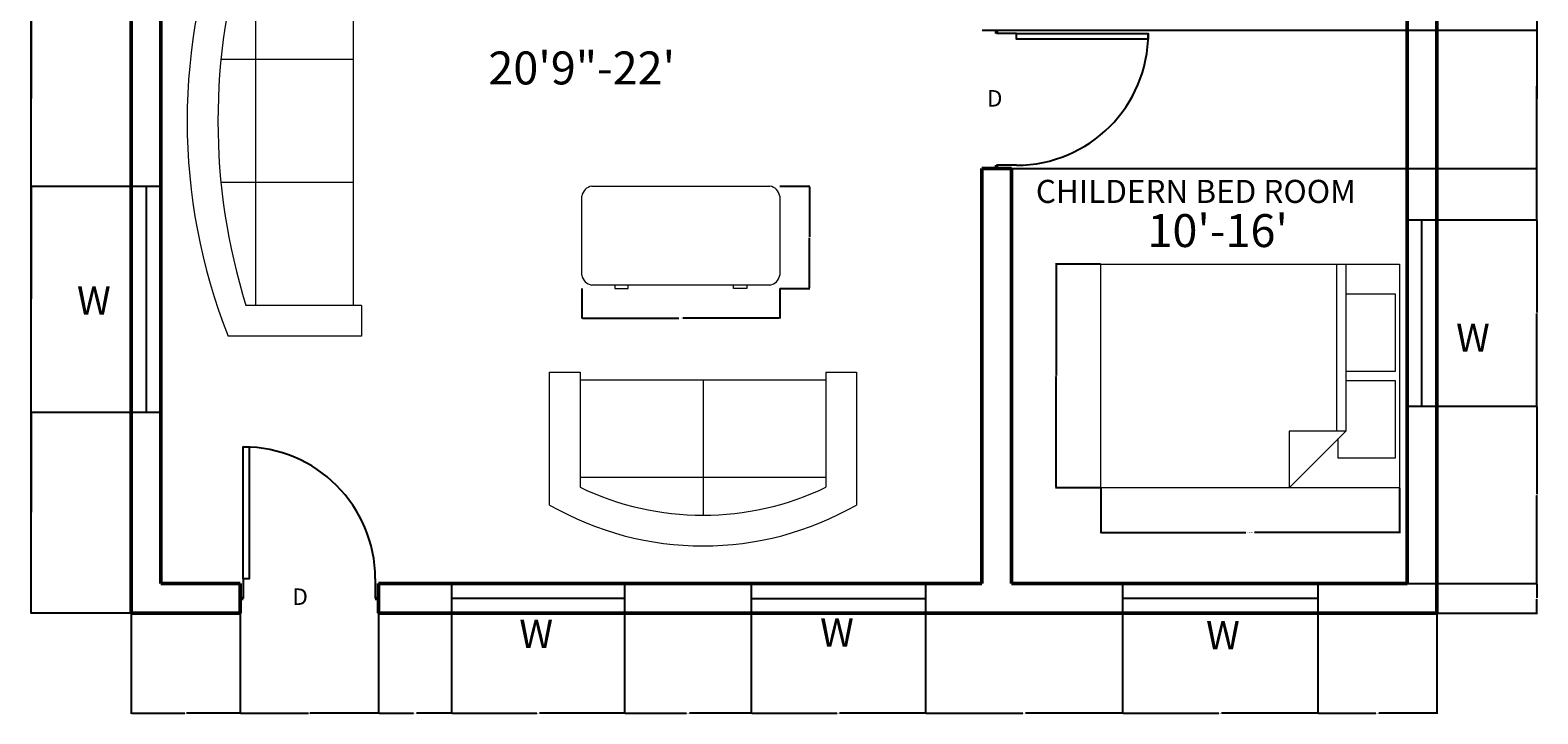
# Model space of a CAD drawing. Units: inches. Extents: x 2164 to 3752, y 2015 to 2629.
# Tile 1 of 8: x 2164 to 2622, y 2015 to 2223. Entities that reach past the tile are written whole.
import ezdxf
from ezdxf.enums import TextEntityAlignment as Align

# ---------------------------------------------------------------- set-up
doc = ezdxf.new("R2010")
doc.units = ezdxf.units.IN
for name, color, linetype, lineweight in [('A-ANNO-DIMS', 2, 'Continuous', 18), ('A-ANNO-TEXT', 7, 'Continuous', 25), ('A-AREA-IDEN', 3, 'Continuous', 25), ('A-DOOR', 3, 'Continuous', 25), ('A-FURN', 8, 'Continuous', 18), ('A-GLAZ', 4, 'Continuous', 25), ('A-WALL', 7, 'Continuous', 50)]:
    doc.layers.add(name, color=color, linetype=linetype, lineweight=lineweight)
doc.styles.get("Standard").update_dxf_attribs({"font": 'arial.ttf'})
doc.dimstyles.get("Standard").update_dxf_attribs({"dimtxt": 0.18, "dimasz": 0.18, "dimexe": 0.18, "dimexo": 0.0625, "dimgap": 0.09, "dimtad": 0, "dimtih": 1, "dimtoh": 1, "dimdec": 4, "dimzin": 0, "dimdsep": 46, "dimtxsty": 'Standard', "dimcen": 0.09, "dimadec": 0, "dimazin": 0, "dimtfac": 1, "dimtdec": 4, "dimtofl": 0, "dimtmove": 0, "dimatfit": 3, "dimfxl": 1, "dimtolj": 1, "dimtzin": 0, "dimarcsym": 0})

# ---------------------------------------------------------------- blocks, each defined once
blk = doc.blocks.new('*U7')
for p, q in [((0, 0), (0, -6)), ((40, 0), (40, -6))]:
    blk.add_line(p, q)
blk.add_lwpolyline([(0, 0), (0, 40), (1.75, 40), (1.75, 0)], close=True)
blk.add_arc((0, 0), 40, 0, 90)
blk = doc.blocks.new('Sofa - Roundback 7 ft.')
for p, q in [((-12.00002, -32.4421), (-12.00003, -6.5971)), ((11.99997, -32.4421), (11.99998, -6.5971)), ((-36.000027, -34), (-36.000027, -11.4696)), ((35.99998, -34), (35.99998, -11.4696)), ((-35.999844, -13.3819), (35.9998, -13.3819)), ((-36.000027, -32.4421), (35.99998, -32.4421))]:
    blk.add_line(p, q)
for points in [[(-36.000027, -34), (-42.000027, -34), (-42.000027, -8)], [(41.99998, -8), (41.99998, -34), (35.99998, -34)]]:
    blk.add_lwpolyline(points)
for centre, radius, start, end in [((0, -114.25), 114.25, 68.43141, 111.5686), ((-0.00001, -127.1968), 121.1968, 72.72033, 107.2797)]:
    blk.add_arc(centre, radius, start, end)
blk = doc.blocks.new('Sofa - Roundback Loveseat 5 ft.')
for p, q in [((0, -32.44198), (0, -5.99998)), ((-24, -33.99998), (-24, -11.46958)), ((24.00004, -33.99998), (24.00004, -11.46958)), ((-23.9998, -13.38178), (23.99986, -13.38178)), ((-24, -32.44198), (24.00004, -32.44198))]:
    blk.add_line(p, q)
for points in [[(-24, -33.99998), (-30, -33.99998), (-30, -7.99998)], [(30.00004, -7.99998), (30.00004, -33.99998), (24.00004, -33.99998)]]:
    blk.add_lwpolyline(points)
for centre, radius, start, end in [((0, -60.24998), 60.24998, 60.13715, 119.8628), ((0, -61.38438), 55.38444, 64.32083, 115.6792)]:
    blk.add_arc(centre, radius, start, end)
blk = doc.blocks.new('Bed - Queen')
for p, q in [((0, -80.00003), (0, 0)), ((0, 0), (59.99999, 0)), ((59.99999, 0), (59.99999, -80.00003)), ((7.99999, -1.2), (28.79998, -1.2)), ((7.99999, -14.4), (7.99999, -1.2)), ((28.79998, -1.2), (28.79998, -14.4)), ((31.19999, -1.2), (51.99999, -1.2)), ((31.19999, -14.4), (31.19999, -1.2)), ((51.99999, -1.2), (51.99999, -16.4)), ((0, -14.4), (44.8, -14.4)), ((59.99999, -29.6), (44.8, -14.4)), ((44.8, -14.4), (44.8, -29.6)), ((44.8, -16.8), (0, -16.8)), ((51.99999, -16.4), (46.79936, -16.4)), ((44.8, -29.6), (59.99999, -29.6)), ((59.99999, -80.00003), (0, -80.00003))]:
    blk.add_line(p, q)
blk = doc.blocks.new('Desk - 30 x 60 in.')
for p, q in [((-26.999995, 0), (26.999995, 0)), ((-29.999995, -27), (-29.999995, -3)), ((29.999995, -3), (29.999995, -27)), ((26.999995, -30), (-26.999995, -30)), ((-20.000005, -30), (-20.000005, -31)), ((-20.000005, -31), (-16.000005, -31)), ((-16.000005, -31), (-16.000005, -30)), ((15.999995, -31), (15.999995, -30)), ((19.999995, -31), (15.999995, -31)), ((19.999995, -30), (19.999995, -31))]:
    blk.add_line(p, q)
for centre, start, end in [((-26.499995, -3.5), 98.1301, 171.8699), ((26.499995, -3.5), 8.130102, 81.8699), ((-26.499995, -26.5), 188.1301, 261.8699), ((26.499995, -26.5), 278.1301, 351.8699)]:
    blk.add_arc(centre, 3.535534, start, end)
blk = doc.blocks.new('*D21')
at = {"layer": 'A-ANNO-DIMS', "color": 0, "lineweight": -2, "transparency": 16777216}
for p, q in [((2489.23, 2083.72), (2489.23, 2070.01)), ((2579.81, 2083.72), (2579.81, 2070.01)), ((2489.41, 2070.19), (2533.21, 2070.19)), ((2579.63, 2070.19), (2535.82, 2070.19))]:
    blk.add_line(p, q, dxfattribs=at)
at = {"layer": 'A-ANNO-DIMS', "color": 0, "transparency": 16777216}
for points in [[(2489.41, 2070.22), (2489.41, 2070.16), (2489.23, 2070.19)], [(2579.63, 2070.22), (2579.63, 2070.16), (2579.81, 2070.19)]]:
    blk.add_solid(points, dxfattribs=at)
at = {"layer": 'Defpoints', "color": 0, "transparency": 16777216}
for p in [(2489.23, 2083.78), (2579.81, 2083.78), (2579.81, 2070.19)]:
    blk.add_point(p, dxfattribs=at)
at = {"layer": 'A-ANNO-DIMS', "color": 0, "transparency": 16777216, "insert": (2534.52, 2070.19), "char_height": 0.18, "attachment_point": 5}
blk.add_mtext('\\A1;QUEEN BED 91 TYP.', dxfattribs=at)
blk = doc.blocks.new('*D22')
at = {"layer": 'A-ANNO-DIMS', "color": 0, "lineweight": -2, "transparency": 16777216}
for p, q in [((2489.16, 2151.72), (2475.46, 2151.72)), ((2475.64, 2151.54), (2475.64, 2117.93)), ((2475.64, 2083.96), (2475.64, 2117.57)), ((2489.16, 2083.78), (2475.46, 2083.78))]:
    blk.add_line(p, q, dxfattribs=at)
at = {"layer": 'A-ANNO-DIMS', "color": 0, "transparency": 16777216}
for points in [[(2475.61, 2151.54), (2475.67, 2151.54), (2475.64, 2151.72)], [(2475.61, 2083.96), (2475.67, 2083.96), (2475.64, 2083.78)]]:
    blk.add_solid(points, dxfattribs=at)
at = {"layer": 'Defpoints', "color": 0, "transparency": 16777216}
for p in [(2489.23, 2151.72), (2475.64, 2083.78), (2489.23, 2083.78)]:
    blk.add_point(p, dxfattribs=at)
at = {"layer": 'A-ANNO-DIMS', "color": 0, "transparency": 16777216, "insert": (2475.64, 2117.75), "char_height": 0.18, "attachment_point": 5}
blk.add_mtext('\\A1;68 TYP.', dxfattribs=at)
blk = doc.blocks.new('*D41')
at = {"layer": 'A-ANNO-DIMS', "color": 0, "lineweight": -2, "transparency": 16777216}
for p, q in [((2331.81, 2144.27), (2331.81, 2135.16)), ((2391.81, 2144.27), (2391.81, 2135.16)), ((2331.99, 2135.34), (2361.22, 2135.34)), ((2391.63, 2135.34), (2362.4, 2135.34))]:
    blk.add_line(p, q, dxfattribs=at)
at = {"layer": 'A-ANNO-DIMS', "color": 0, "transparency": 16777216}
for points in [[(2331.99, 2135.37), (2331.99, 2135.31), (2331.81, 2135.34)], [(2391.63, 2135.37), (2391.63, 2135.31), (2391.81, 2135.34)]]:
    blk.add_solid(points, dxfattribs=at)
at = {"layer": 'Defpoints', "color": 0, "transparency": 16777216}
for p in [(2331.81, 2144.34), (2391.81, 2144.34), (2391.81, 2135.34)]:
    blk.add_point(p, dxfattribs=at)
at = {"layer": 'A-ANNO-DIMS', "color": 0, "transparency": 16777216, "insert": (2361.81, 2135.34), "char_height": 0.18, "attachment_point": 5}
blk.add_mtext('\\A1;DESK 60', dxfattribs=at)
blk = doc.blocks.new('*D42')
at = {"layer": 'A-ANNO-DIMS', "color": 0, "lineweight": -2, "transparency": 16777216}
for p, q in [((2391.87, 2175.34), (2400.99, 2175.34)), ((2400.81, 2175.16), (2400.81, 2160.02)), ((2400.81, 2144.52), (2400.81, 2159.65)), ((2391.87, 2144.34), (2400.99, 2144.34))]:
    blk.add_line(p, q, dxfattribs=at)
at = {"layer": 'A-ANNO-DIMS', "color": 0, "transparency": 16777216}
for points in [[(2400.78, 2175.16), (2400.84, 2175.16), (2400.81, 2175.34)], [(2400.78, 2144.52), (2400.84, 2144.52), (2400.81, 2144.34)]]:
    blk.add_solid(points, dxfattribs=at)
at = {"layer": 'Defpoints', "color": 0, "transparency": 16777216}
for p in [(2391.81, 2175.34), (2400.81, 2175.34), (2391.81, 2144.34)]:
    blk.add_point(p, dxfattribs=at)
at = {"layer": 'A-ANNO-DIMS', "color": 0, "transparency": 16777216, "insert": (2400.81, 2159.84), "char_height": 0.18, "attachment_point": 5}
blk.add_mtext('\\A1;31', dxfattribs=at)
blk = doc.blocks.new('*D59')
at = {"layer": 'A-ANNO-DIMS', "color": 0, "lineweight": -2, "transparency": 16777216}
for p, q in [((2195.11, 2045.65), (2195.11, 2015.19)), ((2228.11, 2045.65), (2228.11, 2015.19)), ((2195.29, 2015.37), (2211.39, 2015.37)), ((2227.93, 2015.37), (2211.83, 2015.37))]:
    blk.add_line(p, q, dxfattribs=at)
at = {"layer": 'A-ANNO-DIMS', "color": 0, "transparency": 16777216}
for points in [[(2195.29, 2015.4), (2195.29, 2015.34), (2195.11, 2015.37)], [(2227.93, 2015.4), (2227.93, 2015.34), (2228.11, 2015.37)]]:
    blk.add_solid(points, dxfattribs=at)
at = {"layer": 'Defpoints', "color": 0, "transparency": 16777216}
for p in [(2195.11, 2045.72), (2228.11, 2045.72), (2228.11, 2015.37)]:
    blk.add_point(p, dxfattribs=at)
at = {"layer": 'A-ANNO-DIMS', "color": 0, "transparency": 16777216, "insert": (2211.61, 2015.37), "char_height": 0.18, "attachment_point": 5}
blk.add_mtext('\\A1;33', dxfattribs=at)
blk = doc.blocks.new('*D60')
at = {"layer": 'A-ANNO-DIMS', "color": 0, "lineweight": -2, "transparency": 16777216}
for p, q in [((2228.11, 2045.65), (2228.11, 2015.19)), ((2270.11, 2045.65), (2270.11, 2015.19)), ((2228.29, 2015.37), (2248.89, 2015.37)), ((2269.93, 2015.37), (2249.33, 2015.37))]:
    blk.add_line(p, q, dxfattribs=at)
at = {"layer": 'A-ANNO-DIMS', "color": 0, "transparency": 16777216}
for points in [[(2228.29, 2015.4), (2228.29, 2015.34), (2228.11, 2015.37)], [(2269.93, 2015.4), (2269.93, 2015.34), (2270.11, 2015.37)]]:
    blk.add_solid(points, dxfattribs=at)
at = {"layer": 'Defpoints', "color": 0, "transparency": 16777216}
for p in [(2228.11, 2045.72), (2270.11, 2045.72), (2270.11, 2015.37)]:
    blk.add_point(p, dxfattribs=at)
at = {"layer": 'A-ANNO-DIMS', "color": 0, "transparency": 16777216, "insert": (2249.11, 2015.37), "char_height": 0.18, "attachment_point": 5}
blk.add_mtext('\\A1;42', dxfattribs=at)
blk = doc.blocks.new('*D61')
at = {"layer": 'A-ANNO-DIMS', "color": 0, "lineweight": -2, "transparency": 16777216}
for p, q in [((2270.11, 2045.65), (2270.11, 2015.19)), ((2292.25, 2045.65), (2292.25, 2015.19)), ((2270.29, 2015.37), (2280.71, 2015.37)), ((2292.07, 2015.37), (2281.64, 2015.37))]:
    blk.add_line(p, q, dxfattribs=at)
at = {"layer": 'A-ANNO-DIMS', "color": 0, "transparency": 16777216}
for points in [[(2270.29, 2015.4), (2270.29, 2015.34), (2270.11, 2015.37)], [(2292.07, 2015.4), (2292.07, 2015.34), (2292.25, 2015.37)]]:
    blk.add_solid(points, dxfattribs=at)
at = {"layer": 'Defpoints', "color": 0, "transparency": 16777216}
for p in [(2270.11, 2045.72), (2292.25, 2045.72), (2292.25, 2015.37)]:
    blk.add_point(p, dxfattribs=at)
at = {"layer": 'A-ANNO-DIMS', "color": 0, "transparency": 16777216, "insert": (2281.18, 2015.37), "char_height": 0.18, "attachment_point": 5}
blk.add_mtext('\\A1;22.137', dxfattribs=at)
blk = doc.blocks.new('*D62')
at = {"layer": 'A-ANNO-DIMS', "color": 0, "lineweight": -2, "transparency": 16777216}
for p, q in [((2292.25, 2045.65), (2292.25, 2015.19)), ((2344.78, 2045.65), (2344.78, 2015.19)), ((2292.43, 2015.37), (2318.12, 2015.37)), ((2344.6, 2015.37), (2318.91, 2015.37))]:
    blk.add_line(p, q, dxfattribs=at)
at = {"layer": 'A-ANNO-DIMS', "color": 0, "transparency": 16777216}
for points in [[(2292.43, 2015.4), (2292.43, 2015.34), (2292.25, 2015.37)], [(2344.6, 2015.4), (2344.6, 2015.34), (2344.78, 2015.37)]]:
    blk.add_solid(points, dxfattribs=at)
at = {"layer": 'Defpoints', "color": 0, "transparency": 16777216}
for p in [(2292.25, 2045.72), (2344.78, 2045.72), (2344.78, 2015.37)]:
    blk.add_point(p, dxfattribs=at)
at = {"layer": 'A-ANNO-DIMS', "color": 0, "transparency": 16777216, "insert": (2318.51, 2015.37), "char_height": 0.18, "attachment_point": 5}
blk.add_mtext('\\A1;52.53', dxfattribs=at)
blk = doc.blocks.new('*D63')
at = {"layer": 'A-ANNO-DIMS', "color": 0, "lineweight": -2, "transparency": 16777216}
for p, q in [((2344.78, 2045.65), (2344.78, 2015.19)), ((2383.15, 2045.65), (2383.15, 2015.19)), ((2344.96, 2015.37), (2363.5, 2015.37)), ((2382.97, 2015.37), (2364.43, 2015.37))]:
    blk.add_line(p, q, dxfattribs=at)
at = {"layer": 'A-ANNO-DIMS', "color": 0, "transparency": 16777216}
for points in [[(2344.96, 2015.4), (2344.96, 2015.34), (2344.78, 2015.37)], [(2382.97, 2015.4), (2382.97, 2015.34), (2383.15, 2015.37)]]:
    blk.add_solid(points, dxfattribs=at)
at = {"layer": 'Defpoints', "color": 0, "transparency": 16777216}
for p in [(2344.78, 2045.72), (2383.15, 2045.72), (2383.15, 2015.37)]:
    blk.add_point(p, dxfattribs=at)
at = {"layer": 'A-ANNO-DIMS', "color": 0, "transparency": 16777216, "insert": (2363.97, 2015.37), "char_height": 0.18, "attachment_point": 5}
blk.add_mtext('\\A1;38.374', dxfattribs=at)
blk = doc.blocks.new('*D64')
at = {"layer": 'A-ANNO-DIMS', "color": 0, "lineweight": -2, "transparency": 16777216}
for p, q in [((2383.15, 2045.65), (2383.15, 2015.19)), ((2436.06, 2045.65), (2436.06, 2015.19)), ((2383.33, 2015.37), (2409.28, 2015.37)), ((2435.88, 2015.37), (2409.93, 2015.37))]:
    blk.add_line(p, q, dxfattribs=at)
at = {"layer": 'A-ANNO-DIMS', "color": 0, "transparency": 16777216}
for points in [[(2383.33, 2015.4), (2383.33, 2015.34), (2383.15, 2015.37)], [(2435.88, 2015.4), (2435.88, 2015.34), (2436.06, 2015.37)]]:
    blk.add_solid(points, dxfattribs=at)
at = {"layer": 'Defpoints', "color": 0, "transparency": 16777216}
for p in [(2383.15, 2045.72), (2436.06, 2045.72), (2436.06, 2015.37)]:
    blk.add_point(p, dxfattribs=at)
at = {"layer": 'A-ANNO-DIMS', "color": 0, "transparency": 16777216, "insert": (2409.61, 2015.37), "char_height": 0.18, "attachment_point": 5}
blk.add_mtext('\\A1;52.9', dxfattribs=at)
blk = doc.blocks.new('*D65')
at = {"layer": 'A-ANNO-DIMS', "color": 0, "lineweight": -2, "transparency": 16777216}
for p, q in [((2436.06, 2045.65), (2436.06, 2015.19)), ((2495.83, 2045.65), (2495.83, 2015.19)), ((2436.24, 2015.37), (2465.55, 2015.37)), ((2495.65, 2015.37), (2466.34, 2015.37))]:
    blk.add_line(p, q, dxfattribs=at)
at = {"layer": 'A-ANNO-DIMS', "color": 0, "transparency": 16777216}
for points in [[(2436.24, 2015.4), (2436.24, 2015.34), (2436.06, 2015.37)], [(2495.65, 2015.4), (2495.65, 2015.34), (2495.83, 2015.37)]]:
    blk.add_solid(points, dxfattribs=at)
at = {"layer": 'Defpoints', "color": 0, "transparency": 16777216}
for p in [(2436.06, 2045.72), (2495.83, 2045.72), (2495.83, 2015.37)]:
    blk.add_point(p, dxfattribs=at)
at = {"layer": 'A-ANNO-DIMS', "color": 0, "transparency": 16777216, "insert": (2465.94, 2015.37), "char_height": 0.18, "attachment_point": 5}
blk.add_mtext('\\A1;59.77', dxfattribs=at)
blk = doc.blocks.new('*D66')
at = {"layer": 'A-ANNO-DIMS', "color": 0, "lineweight": -2, "transparency": 16777216}
for p, q in [((2495.83, 2045.65), (2495.83, 2015.19)), ((2555.02, 2045.65), (2555.02, 2015.19)), ((2496.01, 2015.37), (2525.03, 2015.37)), ((2554.84, 2015.37), (2525.82, 2015.37))]:
    blk.add_line(p, q, dxfattribs=at)
at = {"layer": 'A-ANNO-DIMS', "color": 0, "transparency": 16777216}
for points in [[(2496.01, 2015.4), (2496.01, 2015.34), (2495.83, 2015.37)], [(2554.84, 2015.4), (2554.84, 2015.34), (2555.02, 2015.37)]]:
    blk.add_solid(points, dxfattribs=at)
at = {"layer": 'Defpoints', "color": 0, "transparency": 16777216}
for p in [(2495.83, 2045.72), (2555.02, 2045.72), (2555.02, 2015.37)]:
    blk.add_point(p, dxfattribs=at)
at = {"layer": 'A-ANNO-DIMS', "color": 0, "transparency": 16777216, "insert": (2525.42, 2015.37), "char_height": 0.18, "attachment_point": 5}
blk.add_mtext('\\A1;59.19', dxfattribs=at)
blk = doc.blocks.new('*D67')
at = {"layer": 'A-ANNO-DIMS', "color": 0, "lineweight": -2, "transparency": 16777216}
for p, q in [((2555.02, 2045.65), (2555.02, 2015.19)), ((2591.11, 2045.65), (2591.11, 2015.19)), ((2555.2, 2015.37), (2572.6, 2015.37)), ((2590.93, 2015.37), (2573.53, 2015.37))]:
    blk.add_line(p, q, dxfattribs=at)
at = {"layer": 'A-ANNO-DIMS', "color": 0, "transparency": 16777216}
for points in [[(2555.2, 2015.4), (2555.2, 2015.34), (2555.02, 2015.37)], [(2590.93, 2015.4), (2590.93, 2015.34), (2591.11, 2015.37)]]:
    blk.add_solid(points, dxfattribs=at)
at = {"layer": 'Defpoints', "color": 0, "transparency": 16777216}
for p in [(2555.02, 2045.72), (2591.11, 2045.72), (2591.11, 2015.37)]:
    blk.add_point(p, dxfattribs=at)
at = {"layer": 'A-ANNO-DIMS', "color": 0, "transparency": 16777216, "insert": (2573.06, 2015.37), "char_height": 0.18, "attachment_point": 5}
blk.add_mtext('\\A1;36.096', dxfattribs=at)
blk = doc.blocks.new('*D68')
at = {"layer": 'A-ANNO-DIMS', "color": 0, "lineweight": -2, "transparency": 16777216}
for p, q in [((2195.05, 2106.67), (2164.58, 2106.67)), ((2164.76, 2106.49), (2164.76, 2076.37)), ((2164.76, 2045.9), (2164.76, 2076.01)), ((2195.05, 2045.72), (2164.58, 2045.72))]:
    blk.add_line(p, q, dxfattribs=at)
at = {"layer": 'A-ANNO-DIMS', "color": 0, "transparency": 16777216}
for points in [[(2164.73, 2106.49), (2164.79, 2106.49), (2164.76, 2106.67)], [(2164.73, 2045.9), (2164.79, 2045.9), (2164.76, 2045.72)]]:
    blk.add_solid(points, dxfattribs=at)
at = {"layer": 'Defpoints', "color": 0, "transparency": 16777216}
for p in [(2164.76, 2106.67), (2195.11, 2106.67), (2195.11, 2045.72)]:
    blk.add_point(p, dxfattribs=at)
at = {"layer": 'A-ANNO-DIMS', "color": 0, "transparency": 16777216, "insert": (2164.76, 2076.19), "char_height": 0.18, "attachment_point": 5}
blk.add_mtext('\\A1;60.95', dxfattribs=at)
blk = doc.blocks.new('*D69')
at = {"layer": 'A-ANNO-DIMS', "color": 0, "lineweight": -2, "transparency": 16777216}
for p, q in [((2195.05, 2175.28), (2164.58, 2175.28)), ((2164.76, 2175.1), (2164.76, 2141.16)), ((2164.76, 2106.85), (2164.76, 2140.79)), ((2195.05, 2106.67), (2164.58, 2106.67))]:
    blk.add_line(p, q, dxfattribs=at)
at = {"layer": 'A-ANNO-DIMS', "color": 0, "transparency": 16777216}
for points in [[(2164.73, 2175.1), (2164.79, 2175.1), (2164.76, 2175.28)], [(2164.73, 2106.85), (2164.79, 2106.85), (2164.76, 2106.67)]]:
    blk.add_solid(points, dxfattribs=at)
at = {"layer": 'Defpoints', "color": 0, "transparency": 16777216}
for p in [(2164.76, 2175.28), (2195.11, 2175.28), (2195.11, 2106.67)]:
    blk.add_point(p, dxfattribs=at)
at = {"layer": 'A-ANNO-DIMS', "color": 0, "transparency": 16777216, "insert": (2164.76, 2140.97), "char_height": 0.18, "attachment_point": 5}
blk.add_mtext('\\A1;68.61', dxfattribs=at)
blk = doc.blocks.new('*D70')
at = {"layer": 'A-ANNO-DIMS', "color": 0, "lineweight": -2, "transparency": 16777216}
for p, q in [((2195.05, 2228.35), (2164.58, 2228.35)), ((2164.76, 2228.17), (2164.76, 2202)), ((2164.76, 2175.46), (2164.76, 2201.63)), ((2195.05, 2175.28), (2164.58, 2175.28))]:
    blk.add_line(p, q, dxfattribs=at)
at = {"layer": 'A-ANNO-DIMS', "color": 0, "transparency": 16777216}
for points in [[(2164.73, 2228.17), (2164.79, 2228.17), (2164.76, 2228.35)], [(2164.73, 2175.46), (2164.79, 2175.46), (2164.76, 2175.28)]]:
    blk.add_solid(points, dxfattribs=at)
at = {"layer": 'Defpoints', "color": 0, "transparency": 16777216}
for p in [(2164.76, 2228.35), (2195.11, 2228.35), (2195.11, 2175.28)]:
    blk.add_point(p, dxfattribs=at)
at = {"layer": 'A-ANNO-DIMS', "color": 0, "transparency": 16777216, "insert": (2164.76, 2201.82), "char_height": 0.18, "attachment_point": 5}
blk.add_mtext('\\A1;53.07', dxfattribs=at)
blk = doc.blocks.new('*D75')
at = {"layer": 'A-ANNO-DIMS', "color": 0, "lineweight": -2, "transparency": 16777216}
for p, q in [((2195.05, 2528.72), (2164.58, 2528.72)), ((2164.76, 2528.54), (2164.76, 2287.4)), ((2164.76, 2045.9), (2164.76, 2287.04)), ((2195.05, 2045.72), (2164.58, 2045.72))]:
    blk.add_line(p, q, dxfattribs=at)
at = {"layer": 'A-ANNO-DIMS', "color": 0, "transparency": 16777216}
for points in [[(2164.73, 2528.54), (2164.79, 2528.54), (2164.76, 2528.72)], [(2164.73, 2045.9), (2164.79, 2045.9), (2164.76, 2045.72)]]:
    blk.add_solid(points, dxfattribs=at)
at = {"layer": 'Defpoints', "color": 0, "transparency": 16777216}
for p in [(2164.76, 2528.72), (2195.11, 2528.72), (2195.11, 2045.72)]:
    blk.add_point(p, dxfattribs=at)
at = {"layer": 'A-ANNO-DIMS', "color": 0, "transparency": 16777216, "insert": (2164.76, 2287.22), "char_height": 0.18, "attachment_point": 5}
blk.add_mtext('\\A1;483', dxfattribs=at)
blk = doc.blocks.new('*D76')
at = {"layer": 'A-ANNO-DIMS', "color": 0, "lineweight": -2, "transparency": 16777216}
for p, q in [((2582.17, 2054.72), (2621.64, 2054.72)), ((2621.46, 2054.54), (2621.46, 2050.4)), ((2621.46, 2045.9), (2621.46, 2050.04)), ((2591.17, 2045.72), (2621.64, 2045.72))]:
    blk.add_line(p, q, dxfattribs=at)
at = {"layer": 'A-ANNO-DIMS', "color": 0, "transparency": 16777216}
for points in [[(2621.43, 2054.54), (2621.49, 2054.54), (2621.46, 2054.72)], [(2621.43, 2045.9), (2621.49, 2045.9), (2621.46, 2045.72)]]:
    blk.add_solid(points, dxfattribs=at)
at = {"layer": 'Defpoints', "color": 0, "transparency": 16777216}
for p in [(2582.11, 2054.72), (2621.46, 2054.72), (2591.11, 2045.72)]:
    blk.add_point(p, dxfattribs=at)
at = {"layer": 'A-ANNO-DIMS', "color": 0, "transparency": 16777216, "insert": (2621.46, 2050.22), "char_height": 0.18, "attachment_point": 5}
blk.add_mtext('\\A1;9', dxfattribs=at)
blk = doc.blocks.new('*D77')
at = {"layer": 'A-ANNO-DIMS', "color": 0, "lineweight": -2, "transparency": 16777216}
for p, q in [((2591.17, 2108.58), (2621.64, 2108.58)), ((2621.46, 2108.4), (2621.46, 2081.83)), ((2621.46, 2054.9), (2621.46, 2081.47)), ((2582.17, 2054.72), (2621.64, 2054.72))]:
    blk.add_line(p, q, dxfattribs=at)
at = {"layer": 'A-ANNO-DIMS', "color": 0, "transparency": 16777216}
for points in [[(2621.43, 2108.4), (2621.49, 2108.4), (2621.46, 2108.58)], [(2621.43, 2054.9), (2621.49, 2054.9), (2621.46, 2054.72)]]:
    blk.add_solid(points, dxfattribs=at)
at = {"layer": 'Defpoints', "color": 0, "transparency": 16777216}
for p in [(2591.11, 2108.58), (2621.46, 2108.58), (2582.11, 2054.72)]:
    blk.add_point(p, dxfattribs=at)
at = {"layer": 'A-ANNO-DIMS', "color": 0, "transparency": 16777216, "insert": (2621.46, 2081.65), "char_height": 0.18, "attachment_point": 5}
blk.add_mtext('\\A1;53.86', dxfattribs=at)
blk = doc.blocks.new('*D78')
at = {"layer": 'A-ANNO-DIMS', "color": 0, "lineweight": -2, "transparency": 16777216}
for p, q in [((2591.17, 2165.13), (2621.64, 2165.13)), ((2621.46, 2164.95), (2621.46, 2137.03)), ((2621.46, 2108.76), (2621.46, 2136.67)), ((2591.17, 2108.58), (2621.64, 2108.58))]:
    blk.add_line(p, q, dxfattribs=at)
at = {"layer": 'A-ANNO-DIMS', "color": 0, "transparency": 16777216}
for points in [[(2621.43, 2164.95), (2621.49, 2164.95), (2621.46, 2165.13)], [(2621.43, 2108.76), (2621.49, 2108.76), (2621.46, 2108.58)]]:
    blk.add_solid(points, dxfattribs=at)
at = {"layer": 'Defpoints', "color": 0, "transparency": 16777216}
for p in [(2591.11, 2165.13), (2621.46, 2165.13), (2591.11, 2108.58)]:
    blk.add_point(p, dxfattribs=at)
at = {"layer": 'A-ANNO-DIMS', "color": 0, "transparency": 16777216, "insert": (2621.46, 2136.85), "char_height": 0.18, "attachment_point": 5}
blk.add_mtext('\\A1;56.55', dxfattribs=at)
blk = doc.blocks.new('*D79')
at = {"layer": 'A-ANNO-DIMS', "color": 0, "lineweight": -2, "transparency": 16777216}
for p, q in [((2582.17, 2246.72), (2621.64, 2246.72)), ((2621.46, 2246.54), (2621.46, 2206.1)), ((2621.46, 2165.31), (2621.46, 2205.74)), ((2591.17, 2165.13), (2621.64, 2165.13))]:
    blk.add_line(p, q, dxfattribs=at)
at = {"layer": 'A-ANNO-DIMS', "color": 0, "transparency": 16777216}
for points in [[(2621.43, 2246.54), (2621.49, 2246.54), (2621.46, 2246.72)], [(2621.43, 2165.31), (2621.49, 2165.31), (2621.46, 2165.13)]]:
    blk.add_solid(points, dxfattribs=at)
at = {"layer": 'Defpoints', "color": 0, "transparency": 16777216}
for p in [(2582.11, 2246.72), (2621.46, 2246.72), (2591.11, 2165.13)]:
    blk.add_point(p, dxfattribs=at)
at = {"layer": 'A-ANNO-DIMS', "color": 0, "transparency": 16777216, "insert": (2621.46, 2205.92), "char_height": 0.18, "attachment_point": 5}
blk.add_mtext('\\A1;81.59', dxfattribs=at)
blk = doc.blocks.new('*D98')
at = {"layer": 'A-ANNO-DIMS', "color": 0, "lineweight": -2, "transparency": 16777216}
for p, q in [((2453.17, 2222.72), (2621.64, 2222.72)), ((2621.46, 2222.54), (2621.46, 2201.9)), ((2621.46, 2180.9), (2621.46, 2201.54)), ((2453.17, 2180.72), (2621.64, 2180.72))]:
    blk.add_line(p, q, dxfattribs=at)
at = {"layer": 'A-ANNO-DIMS', "color": 0, "transparency": 16777216}
for points in [[(2621.43, 2222.54), (2621.49, 2222.54), (2621.46, 2222.72)], [(2621.43, 2180.9), (2621.49, 2180.9), (2621.46, 2180.72)]]:
    blk.add_solid(points, dxfattribs=at)
at = {"layer": 'Defpoints', "color": 0, "transparency": 16777216}
for p in [(2453.11, 2222.72), (2621.46, 2222.72), (2453.11, 2180.72)]:
    blk.add_point(p, dxfattribs=at)
at = {"layer": 'A-ANNO-DIMS', "color": 0, "transparency": 16777216, "insert": (2621.46, 2201.72), "char_height": 0.18, "attachment_point": 5}
blk.add_mtext('\\A1;42', dxfattribs=at)

msp = doc.modelspace()

# ---------------------------------------------------------------- linework, layer by layer
at = {"layer": 'A-GLAZ'}
for p, q in [((2204.1113, 2175.28), (2195.1113, 2175.28)), ((2199.6113, 2175.28), (2199.6113, 2106.6668)), ((2582.1113, 2165.1259), (2591.1113, 2165.1259)), ((2586.6113, 2108.5768), (2586.6113, 2165.1259)), ((2582.1113, 2108.5768), (2591.1113, 2108.5768)), ((2204.1113, 2106.6668), (2195.1113, 2106.6668)), ((2292.2479, 2054.7172), (2292.2479, 2045.7172)), ((2344.7797, 2054.7172), (2344.7797, 2045.7172)), ((2383.154, 2054.7172), (2383.154, 2045.7172)), ((2436.0584, 2054.7172), (2436.0584, 2045.7172)), ((2495.8302, 2054.7172), (2495.8302, 2045.7172)), ((2555.0152, 2054.7172), (2555.0152, 2045.7172)), ((2344.7797, 2050.2172), (2292.2479, 2050.2172)), ((2383.154, 2050.2172), (2436.0584, 2050.2172)), ((2555.0152, 2050.2172), (2495.8302, 2050.2172))]:
    msp.add_line(p, q, dxfattribs=at)
at = {"layer": 'A-WALL'}
for p, q in [((2195.1113, 2528.7172), (2195.1113, 2045.7172)), ((2591.1113, 2528.7172), (2591.1113, 2045.7172)), ((2204.1113, 2318.7172), (2204.1113, 2054.7172)), ((2582.1113, 2318.7172), (2582.1113, 2054.7172)), ((2457.6113, 2222.7172), (2457.6113, 2221.7172)), ((2457.6113, 2181.7172), (2457.6113, 2180.7172)), ((2453.1113, 2180.7172), (2453.1113, 2054.7172)), ((2457.6113, 2180.7172), (2453.1113, 2180.7172)), ((2457.6113, 2180.7172), (2462.1113, 2180.7172)), ((2462.1113, 2180.7172), (2462.1113, 2054.7172)), ((2204.1113, 2054.7172), (2228.1113, 2054.7172)), ((2228.1113, 2054.7172), (2228.1113, 2045.7172)), ((2270.1113, 2054.7172), (2453.1113, 2054.7172)), ((2270.1113, 2050.2172), (2270.1113, 2054.7172)), ((2381.1113, 2054.7172), (2453.1113, 2054.7172)), ((2462.1113, 2054.7172), (2582.1113, 2054.7172)), ((2228.1113, 2050.2172), (2229.1113, 2050.2172)), ((2269.1113, 2050.2172), (2270.1113, 2050.2172)), ((2270.1113, 2050.2172), (2270.1113, 2045.7172)), ((2195.1113, 2045.7172), (2228.1113, 2045.7172)), ((2270.1113, 2045.7172), (2591.1113, 2045.7172))]:
    msp.add_line(p, q, dxfattribs=at)

# ---------------------------------------------------------------- block references
at = {"layer": 'A-DOOR', "rotation": 270}
msp.add_blockref('*U7', (2463.6113, 2221.7172), dxfattribs=at)
at = {"layer": 'A-DOOR'}
msp.add_blockref('*U7', (2229.1113, 2056.2172), dxfattribs=at)
at = {"layer": 'A-FURN'}
for name, p, xscale, yscale, zscale, rotation in [('Sofa - Roundback 7 ft.', (2212.0723, 2195.1336), 1.554837866346122, 1.554837866346122, 1.554837866346122, 90), ('Bed - Queen', (2579.8096, 2151.7177), 1.1322848164304, 1.1322848164304, 1.1322848164304, 270), ('Sofa - Roundback Loveseat 5 ft.', (2368.5435, 2066.1683), 1.550400962032466, 1.550400962032466, 1.550400962032466, 180)]:
    msp.add_blockref(name, p, dxfattribs=dict(at, xscale=xscale, yscale=yscale, zscale=zscale, rotation=rotation))
msp.add_blockref('Desk - 30 x 60 in.', (2361.812, 2175.3369), dxfattribs=at)

# ---------------------------------------------------------------- texts
at = {"layer": 'A-ANNO-TEXT'}
for p in [(2454.673, 2199.5141), (2244.0093, 2048.252)]:
    msp.add_text('D', height=5, dxfattribs=at).set_placement(p)
for p in [(2183.7849, 2139.525), (2602.0802, 2128.2853), (2317.9393, 2038.3677), (2409.1811, 2038.784), (2526.2538, 2037.9514)]:
    msp.add_text('W', height=8.5558, dxfattribs=at).set_placement(p, align=Align.MIDDLE)
at = {"layer": 'A-AREA-IDEN'}
for s, height, p in [('20\'9"-22\'', 10, (2303.441, 2206.2404)), ('CHILDERN BED ROOM', 7.006737, (2469.5042, 2170.2644)), ("10'-16'", 10, (2503.3609, 2156.8789))]:
    msp.add_text(s, height=height, dxfattribs=at).set_placement(p)

# ---------------------------------------------------------------- dimensions: what is measured, and where the dimension line sits
at = {"layer": 'A-ANNO-DIMS'}
for base, p1, p2, override, picture, middle in [((2164.7613, 2528.7172), (2195.1113, 2045.7172), (2195.1113, 2528.7172), {"dimdec": 0, "dimlfac": 1, "dimrnd": 0, "dimzin": 0, "dimdsep": 46, "dimlunit": 2}, '*D75', (2164.7613, 2287.2172)), ((2621.4613, 2246.7172), (2591.1113, 2165.1259), (2582.1113, 2246.7172), {"dimdec": 2, "dimlfac": 1, "dimrnd": 0, "dimzin": 0, "dimdsep": 46, "dimlunit": 2}, '*D79', (2621.4613, 2205.9216)), ((2164.7613, 2228.3505), (2195.1113, 2175.28), (2195.1113, 2228.3505), {"dimdec": 2, "dimlfac": 1, "dimrnd": 0, "dimzin": 0, "dimdsep": 46, "dimlunit": 2}, '*D70', (2164.7613, 2201.8152)), ((2621.4613, 2222.7172), (2453.1113, 2180.7172), (2453.1113, 2222.7172), {"dimdec": 0, "dimlfac": 1, "dimrnd": 0, "dimzin": 0, "dimdsep": 46, "dimlunit": 2}, '*D98', (2621.4613, 2201.7172)), ((2164.7613, 2175.28), (2195.1113, 2106.6668), (2195.1113, 2175.28), {"dimdec": 2, "dimlfac": 1, "dimrnd": 0, "dimzin": 0, "dimdsep": 46, "dimlunit": 2}, '*D69', (2164.7613, 2140.9734)), ((2400.812, 2175.3369), (2391.812, 2144.3369), (2391.812, 2175.3369), {"dimdec": 0, "dimrnd": 0, "dimzin": 0, "dimlunit": 2}, '*D42', (2400.812, 2159.8369)), ((2621.4613, 2165.1259), (2591.1113, 2108.5768), (2591.1113, 2165.1259), {"dimdec": 2, "dimlfac": 1, "dimrnd": 0, "dimzin": 0, "dimdsep": 46, "dimlunit": 2}, '*D78', (2621.4613, 2136.8514)), ((2621.4613, 2108.5768), (2582.1113, 2054.7172), (2591.1113, 2108.5768), {"dimdec": 2, "dimlfac": 1, "dimrnd": 0, "dimzin": 0, "dimdsep": 46, "dimlunit": 2}, '*D77', (2621.4613, 2081.647)), ((2164.7613, 2106.6668), (2195.1113, 2045.7172), (2195.1113, 2106.6668), {"dimdec": 2, "dimlfac": 1, "dimrnd": 0, "dimzin": 0, "dimdsep": 46, "dimlunit": 2}, '*D68', (2164.7613, 2076.192)), ((2621.4613, 2054.7172), (2591.1113, 2045.7172), (2582.1113, 2054.7172), {"dimdec": 0, "dimlfac": 1, "dimrnd": 0, "dimzin": 0, "dimdsep": 46, "dimlunit": 2}, '*D76', (2621.4613, 2050.2172))]:
    dim = msp.add_linear_dim(base=base, p1=p1, p2=p2, angle=90, dimstyle='Standard', override=override, dxfattribs=at)
    dim.commit()
    dim.dimension.update_dxf_attribs({"geometry": picture, "text_midpoint": middle})
dim = msp.add_linear_dim(base=(2475.6394, 2083.7806), p1=(2489.2268, 2151.7177), p2=(2489.2268, 2083.7806), angle=270, text='<> TYP.', dimstyle='Standard', override={"dimdec": 0, "dimrnd": 0, "dimzin": 0, "dimlunit": 2}, dxfattribs=at)
dim.commit()
dim.dimension.update_dxf_attribs({"geometry": '*D22', "text_midpoint": (2475.6394, 2117.7492)})
for base, p1, p2, text, picture, middle in [((2391.812, 2135.3369), (2331.8121, 2144.3369), (2391.812, 2144.3369), 'DESK <>', '*D41', (2361.812, 2135.3369)), ((2579.8096, 2070.1932), (2489.2268, 2083.7806), (2579.8096, 2083.7806), 'QUEEN BED <> TYP.', '*D21', (2534.5182, 2070.1932))]:
    dim = msp.add_linear_dim(base=base, p1=p1, p2=p2, text=text, dimstyle='Standard', override={"dimdec": 0, "dimrnd": 0, "dimzin": 0, "dimlunit": 2}, dxfattribs=at)
    dim.commit()
    dim.dimension.update_dxf_attribs({"geometry": picture, "text_midpoint": middle})
for base, p1, p2, override, picture, middle in [((2228.1113, 2015.3672), (2195.1113, 2045.7172), (2228.1113, 2045.7172), {"dimdec": 0, "dimlfac": 1, "dimrnd": 0, "dimzin": 0, "dimdsep": 46, "dimlunit": 2}, '*D59', (2211.6113, 2015.3672)), ((2270.1113, 2015.3672), (2228.1113, 2045.7172), (2270.1113, 2045.7172), {"dimdec": 0, "dimlfac": 1, "dimrnd": 0, "dimzin": 0, "dimdsep": 46, "dimlunit": 2}, '*D60', (2249.1113, 2015.3672)), ((2292.2479, 2015.3672), (2270.1113, 2045.7172), (2292.2479, 2045.7172), {"dimdec": 3, "dimlfac": 1, "dimrnd": 0, "dimzin": 0, "dimdsep": 46, "dimlunit": 2}, '*D61', (2281.1796, 2015.3672)), ((2344.7797, 2015.3672), (2292.2479, 2045.7172), (2344.7797, 2045.7172), {"dimdec": 2, "dimlfac": 1, "dimrnd": 0, "dimzin": 0, "dimdsep": 46, "dimlunit": 2}, '*D62', (2318.5138, 2015.3672)), ((2383.154, 2015.3672), (2344.7797, 2045.7172), (2383.154, 2045.7172), {"dimdec": 3, "dimlfac": 1, "dimrnd": 0, "dimzin": 0, "dimdsep": 46, "dimlunit": 2}, '*D63', (2363.9668, 2015.3672)), ((2436.0584, 2015.3672), (2383.154, 2045.7172), (2436.0584, 2045.7172), {"dimdec": 1, "dimlfac": 1, "dimrnd": 0, "dimzin": 0, "dimdsep": 46, "dimlunit": 2}, '*D64', (2409.6062, 2015.3672)), ((2495.8302, 2015.3672), (2436.0584, 2045.7172), (2495.8302, 2045.7172), {"dimdec": 2, "dimlfac": 1, "dimrnd": 0, "dimzin": 0, "dimdsep": 46, "dimlunit": 2}, '*D65', (2465.9443, 2015.3672)), ((2555.01523, 2015.36725), (2495.83017, 2045.71725), (2555.01523, 2045.71725), {"dimdec": 2, "dimlfac": 1, "dimrnd": 0, "dimzin": 0, "dimdsep": 46, "dimlunit": 2}, '*D66', (2525.4227, 2015.36725)), ((2591.1113, 2015.3672), (2555.0152, 2045.7172), (2591.1113, 2045.7172), {"dimdec": 3, "dimlfac": 1, "dimrnd": 0, "dimzin": 0, "dimdsep": 46, "dimlunit": 2}, '*D67', (2573.0633, 2015.3672))]:
    dim = msp.add_linear_dim(base=base, p1=p1, p2=p2, dimstyle='Standard', override=override, dxfattribs=at)
    dim.commit()
    dim.dimension.update_dxf_attribs({"geometry": picture, "text_midpoint": middle})

doc.saveas('drawing.dxf')
